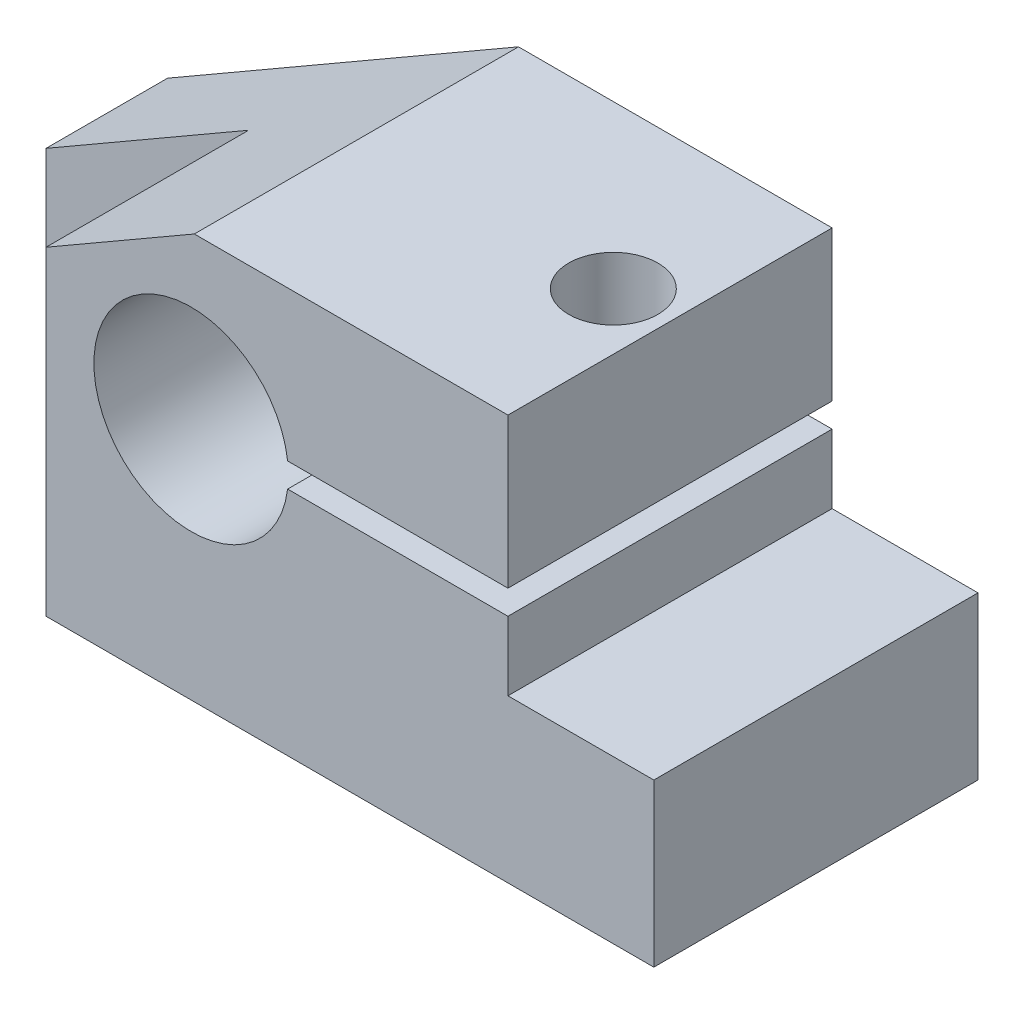
ISO-10303-21;
HEADER;
FILE_DESCRIPTION(('STEP AP214'),'2;1');
FILE_NAME('part.step','',(''),(''),'','','');
FILE_SCHEMA(('AUTOMOTIVE_DESIGN { 1 0 10303 214 1 1 1 1 }'));
ENDSEC;
DATA;
#1=APPLICATION_CONTEXT('core data for automotive mechanical design processes');
#2=APPLICATION_PROTOCOL_DEFINITION('international standard','automotive_design',2000,#1);
#3=PRODUCT_CONTEXT('',#1,'mechanical');
#4=PRODUCT('Part','Part','',(#3));
#5=PRODUCT_RELATED_PRODUCT_CATEGORY('part','',(#4));
#6=PRODUCT_DEFINITION_FORMATION('','',#4);
#7=PRODUCT_DEFINITION_CONTEXT('part definition',#1,'design');
#8=PRODUCT_DEFINITION('design','',#6,#7);
#9=PRODUCT_DEFINITION_SHAPE('','',#8);
#10=(LENGTH_UNIT() NAMED_UNIT(*) SI_UNIT(.MILLI.,.METRE.));
#11=(NAMED_UNIT(*) PLANE_ANGLE_UNIT() SI_UNIT($,.RADIAN.));
#12=(NAMED_UNIT(*) SI_UNIT($,.STERADIAN.) SOLID_ANGLE_UNIT());
#13=UNCERTAINTY_MEASURE_WITH_UNIT(LENGTH_MEASURE(1.E-05),#10,'distance_accuracy_value','');
#14=(GEOMETRIC_REPRESENTATION_CONTEXT(3) GLOBAL_UNCERTAINTY_ASSIGNED_CONTEXT((#13)) GLOBAL_UNIT_ASSIGNED_CONTEXT((#10,
#11,#12)) REPRESENTATION_CONTEXT('',''));
#15=CARTESIAN_POINT('',(0.,0.,0.));
#16=DIRECTION('',(0.,0.,1.));
#17=DIRECTION('',(1.,0.,0.));
#18=AXIS2_PLACEMENT_3D('',#15,#16,#17);
#19=CARTESIAN_POINT('',(-58.3395488539924,25.,40.));
#20=DIRECTION('',(1.,0.,0.));
#21=DIRECTION('',(0.,0.,-1.));
#22=AXIS2_PLACEMENT_3D('',#19,#20,#21);
#23=PLANE('',#22);
#24=DIRECTION('',(0.,0.,-1.));
#25=VECTOR('',#24,1.);
#26=CARTESIAN_POINT('',(-58.3395488539924,0.,40.));
#27=LINE('',#26,#25);
#28=CARTESIAN_POINT('',(-58.3395488539924,0.,15.));
#29=VERTEX_POINT('',#28);
#30=CARTESIAN_POINT('',(-58.3395488539924,0.,0.));
#31=VERTEX_POINT('',#30);
#32=EDGE_CURVE('E11',#29,#31,#27,.T.);
#33=ORIENTED_EDGE('',*,*,#32,.F.);
#34=DIRECTION('',(0.,-1.,0.));
#35=VECTOR('',#34,1.);
#36=CARTESIAN_POINT('',(-58.3395488539924,50.,15.));
#37=LINE('',#36,#35);
#38=CARTESIAN_POINT('',(-58.3395488539924,25.,15.));
#39=VERTEX_POINT('',#38);
#40=EDGE_CURVE('E257',#39,#29,#37,.T.);
#41=ORIENTED_EDGE('',*,*,#40,.F.);
#42=DIRECTION('',(0.,0.,-1.));
#43=VECTOR('',#42,1.);
#44=CARTESIAN_POINT('',(-58.3395488539924,25.,40.));
#45=LINE('',#44,#43);
#46=CARTESIAN_POINT('',(-58.3395488539924,25.,0.));
#47=VERTEX_POINT('',#46);
#48=EDGE_CURVE('E110',#39,#47,#45,.T.);
#49=ORIENTED_EDGE('',*,*,#48,.T.);
#50=DIRECTION('',(0.,-1.,0.));
#51=VECTOR('',#50,1.);
#52=CARTESIAN_POINT('',(-58.3395488539924,25.,0.));
#53=LINE('',#52,#51);
#54=EDGE_CURVE('E164',#47,#31,#53,.T.);
#55=ORIENTED_EDGE('',*,*,#54,.T.);
#56=EDGE_LOOP('',(#33,#41,#49,#55));
#57=FACE_BOUND('',#56,.T.);
#58=ADVANCED_FACE('F41',(#57),#23,.F.);
#59=CARTESIAN_POINT('',(-58.3395488539924,0.,40.));
#60=DIRECTION('',(0.,1.,0.));
#61=DIRECTION('',(0.,0.,1.));
#62=AXIS2_PLACEMENT_3D('',#59,#60,#61);
#63=PLANE('',#62);
#64=DIRECTION('',(1.,0.,0.));
#65=VECTOR('',#64,1.);
#66=CARTESIAN_POINT('',(-58.3395488539924,0.,40.));
#67=LINE('',#66,#65);
#68=CARTESIAN_POINT('',(-33.3395488539924,0.,40.));
#69=VERTEX_POINT('',#68);
#70=CARTESIAN_POINT('',(41.6604511460076,0.,40.));
#71=VERTEX_POINT('',#70);
#72=EDGE_CURVE('E113',#69,#71,#67,.T.);
#73=ORIENTED_EDGE('',*,*,#72,.F.);
#74=DIRECTION('',(0.,0.,1.));
#75=VECTOR('',#74,1.);
#76=CARTESIAN_POINT('',(-33.3395488539924,0.,15.));
#77=LINE('',#76,#75);
#78=CARTESIAN_POINT('',(-33.3395488539924,0.,15.));
#79=VERTEX_POINT('',#78);
#80=EDGE_CURVE('E57',#79,#69,#77,.T.);
#81=ORIENTED_EDGE('',*,*,#80,.F.);
#82=DIRECTION('',(1.,0.,0.));
#83=VECTOR('',#82,1.);
#84=CARTESIAN_POINT('',(-58.3395488539924,0.,15.));
#85=LINE('',#84,#83);
#86=EDGE_CURVE('E262',#29,#79,#85,.T.);
#87=ORIENTED_EDGE('',*,*,#86,.F.);
#88=ORIENTED_EDGE('',*,*,#32,.T.);
#89=DIRECTION('',(1.,0.,0.));
#90=VECTOR('',#89,1.);
#91=CARTESIAN_POINT('',(-58.3395488539924,0.,0.));
#92=LINE('',#91,#90);
#93=CARTESIAN_POINT('',(41.6604511460076,0.,0.));
#94=VERTEX_POINT('',#93);
#95=EDGE_CURVE('E170',#31,#94,#92,.T.);
#96=ORIENTED_EDGE('',*,*,#95,.T.);
#97=DIRECTION('',(0.,0.,-1.));
#98=VECTOR('',#97,1.);
#99=CARTESIAN_POINT('',(41.6604511460076,0.,40.));
#100=LINE('',#99,#98);
#101=EDGE_CURVE('E47',#71,#94,#100,.T.);
#102=ORIENTED_EDGE('',*,*,#101,.F.);
#103=EDGE_LOOP('',(#73,#81,#87,#88,#96,#102));
#104=FACE_BOUND('',#103,.T.);
#105=ADVANCED_FACE('F269',(#104),#63,.F.);
#106=CARTESIAN_POINT('',(41.6604511460076,0.,40.));
#107=DIRECTION('',(-1.,0.,0.));
#108=DIRECTION('',(0.,0.,1.));
#109=AXIS2_PLACEMENT_3D('',#106,#107,#108);
#110=PLANE('',#109);
#111=DIRECTION('',(0.,1.,0.));
#112=VECTOR('',#111,1.);
#113=CARTESIAN_POINT('',(41.6604511460076,0.,0.));
#114=LINE('',#113,#112);
#115=CARTESIAN_POINT('',(41.6604511460076,20.,0.));
#116=VERTEX_POINT('',#115);
#117=EDGE_CURVE('E168',#94,#116,#114,.T.);
#118=ORIENTED_EDGE('',*,*,#117,.T.);
#119=DIRECTION('',(0.,0.,-1.));
#120=VECTOR('',#119,1.);
#121=CARTESIAN_POINT('',(41.6604511460076,20.,40.));
#122=LINE('',#121,#120);
#123=CARTESIAN_POINT('',(41.6604511460076,20.,40.));
#124=VERTEX_POINT('',#123);
#125=EDGE_CURVE('E204',#124,#116,#122,.T.);
#126=ORIENTED_EDGE('',*,*,#125,.F.);
#127=DIRECTION('',(0.,1.,0.));
#128=VECTOR('',#127,1.);
#129=CARTESIAN_POINT('',(41.6604511460076,0.,40.));
#130=LINE('',#129,#128);
#131=EDGE_CURVE('E213',#71,#124,#130,.T.);
#132=ORIENTED_EDGE('',*,*,#131,.F.);
#133=ORIENTED_EDGE('',*,*,#101,.T.);
#134=EDGE_LOOP('',(#118,#126,#132,#133));
#135=FACE_BOUND('',#134,.T.);
#136=ADVANCED_FACE('F211',(#135),#110,.F.);
#137=CARTESIAN_POINT('',(41.6604511460076,20.,40.));
#138=DIRECTION('',(0.,-1.,0.));
#139=DIRECTION('',(0.,0.,-1.));
#140=AXIS2_PLACEMENT_3D('',#137,#138,#139);
#141=PLANE('',#140);
#142=DIRECTION('',(-1.,0.,0.));
#143=VECTOR('',#142,1.);
#144=CARTESIAN_POINT('',(41.6604511460076,20.,0.));
#145=LINE('',#144,#143);
#146=CARTESIAN_POINT('',(23.6604511460076,20.,0.));
#147=VERTEX_POINT('',#146);
#148=EDGE_CURVE('E175',#116,#147,#145,.T.);
#149=ORIENTED_EDGE('',*,*,#148,.T.);
#150=DIRECTION('',(0.,0.,-1.));
#151=VECTOR('',#150,1.);
#152=CARTESIAN_POINT('',(23.6604511460076,20.,40.));
#153=LINE('',#152,#151);
#154=CARTESIAN_POINT('',(23.6604511460076,20.,40.));
#155=VERTEX_POINT('',#154);
#156=EDGE_CURVE('E203',#155,#147,#153,.T.);
#157=ORIENTED_EDGE('',*,*,#156,.F.);
#158=DIRECTION('',(-1.,0.,0.));
#159=VECTOR('',#158,1.);
#160=CARTESIAN_POINT('',(41.6604511460076,20.,40.));
#161=LINE('',#160,#159);
#162=EDGE_CURVE('E232',#124,#155,#161,.T.);
#163=ORIENTED_EDGE('',*,*,#162,.F.);
#164=ORIENTED_EDGE('',*,*,#125,.T.);
#165=EDGE_LOOP('',(#149,#157,#163,#164));
#166=FACE_BOUND('',#165,.T.);
#167=ADVANCED_FACE('F224',(#166),#141,.F.);
#168=CARTESIAN_POINT('',(23.6604511460076,20.,40.));
#169=DIRECTION('',(-1.,0.,0.));
#170=DIRECTION('',(0.,0.,1.));
#171=AXIS2_PLACEMENT_3D('',#168,#169,#170);
#172=PLANE('',#171);
#173=DIRECTION('',(0.,1.,0.));
#174=VECTOR('',#173,1.);
#175=CARTESIAN_POINT('',(23.6604511460076,20.,0.));
#176=LINE('',#175,#174);
#177=CARTESIAN_POINT('',(23.6604511460076,28.5,0.));
#178=VERTEX_POINT('',#177);
#179=EDGE_CURVE('E174',#147,#178,#176,.T.);
#180=ORIENTED_EDGE('',*,*,#179,.T.);
#181=DIRECTION('',(0.,0.,-1.));
#182=VECTOR('',#181,1.);
#183=CARTESIAN_POINT('',(23.6604511460076,28.5,40.));
#184=LINE('',#183,#182);
#185=CARTESIAN_POINT('',(23.6604511460076,28.5,40.));
#186=VERTEX_POINT('',#185);
#187=EDGE_CURVE('E196',#186,#178,#184,.T.);
#188=ORIENTED_EDGE('',*,*,#187,.F.);
#189=DIRECTION('',(0.,1.,0.));
#190=VECTOR('',#189,1.);
#191=CARTESIAN_POINT('',(23.6604511460076,20.,40.));
#192=LINE('',#191,#190);
#193=EDGE_CURVE('E229',#155,#186,#192,.T.);
#194=ORIENTED_EDGE('',*,*,#193,.F.);
#195=ORIENTED_EDGE('',*,*,#156,.T.);
#196=EDGE_LOOP('',(#180,#188,#194,#195));
#197=FACE_BOUND('',#196,.T.);
#198=ADVANCED_FACE('F230',(#197),#172,.F.);
#199=CARTESIAN_POINT('',(23.6604511460076,28.5,40.));
#200=DIRECTION('',(0.,-1.,0.));
#201=DIRECTION('',(1.,0.,0.));
#202=AXIS2_PLACEMENT_3D('',#199,#200,#201);
#203=PLANE('',#202);
#204=DIRECTION('',(-1.,0.,0.));
#205=VECTOR('',#204,1.);
#206=CARTESIAN_POINT('',(23.6604511460076,28.5,0.));
#207=LINE('',#206,#205);
#208=CARTESIAN_POINT('',(-3.52361977982805,28.5,0.));
#209=VERTEX_POINT('',#208);
#210=EDGE_CURVE('E176',#178,#209,#207,.T.);
#211=ORIENTED_EDGE('',*,*,#210,.T.);
#212=DIRECTION('',(0.,0.,-1.));
#213=VECTOR('',#212,1.);
#214=CARTESIAN_POINT('',(-3.52361977982805,28.5,40.));
#215=LINE('',#214,#213);
#216=CARTESIAN_POINT('',(-3.52361977982805,28.5,40.));
#217=VERTEX_POINT('',#216);
#218=EDGE_CURVE('E198',#217,#209,#215,.T.);
#219=ORIENTED_EDGE('',*,*,#218,.F.);
#220=DIRECTION('',(-1.,0.,0.));
#221=VECTOR('',#220,1.);
#222=CARTESIAN_POINT('',(23.6604511460076,28.5,40.));
#223=LINE('',#222,#221);
#224=EDGE_CURVE('E231',#186,#217,#223,.T.);
#225=ORIENTED_EDGE('',*,*,#224,.F.);
#226=ORIENTED_EDGE('',*,*,#187,.T.);
#227=EDGE_LOOP('',(#211,#219,#225,#226));
#228=FACE_BOUND('',#227,.T.);
#229=ADVANCED_FACE('F313',(#228),#203,.F.);
#230=CARTESIAN_POINT('',(-15.4295006796187,30.,40.));
#231=DIRECTION('',(0.,0.,-1.));
#232=DIRECTION('',(-1.,0.,0.));
#233=AXIS2_PLACEMENT_3D('',#230,#231,#232);
#234=CYLINDRICAL_SURFACE('',#233,12.);
#235=CARTESIAN_POINT('',(-15.4295006796187,30.,0.));
#236=DIRECTION('',(0.,0.,1.));
#237=DIRECTION('',(1.,0.,0.));
#238=AXIS2_PLACEMENT_3D('',#235,#236,#237);
#239=CIRCLE('',#238,12.);
#240=CARTESIAN_POINT('',(-3.52361977982805,31.5,0.));
#241=VERTEX_POINT('',#240);
#242=EDGE_CURVE('E178',#241,#209,#239,.T.);
#243=ORIENTED_EDGE('',*,*,#242,.F.);
#244=DIRECTION('',(0.,0.,-1.));
#245=VECTOR('',#244,1.);
#246=CARTESIAN_POINT('',(-3.52361977982805,31.5,40.));
#247=LINE('',#246,#245);
#248=CARTESIAN_POINT('',(-3.52361977982805,31.5,40.));
#249=VERTEX_POINT('',#248);
#250=EDGE_CURVE('E152',#249,#241,#247,.T.);
#251=ORIENTED_EDGE('',*,*,#250,.F.);
#252=CARTESIAN_POINT('',(-15.4295006796187,30.,40.));
#253=DIRECTION('',(0.,0.,1.));
#254=DIRECTION('',(1.,0.,0.));
#255=AXIS2_PLACEMENT_3D('',#252,#253,#254);
#256=CIRCLE('',#255,12.);
#257=EDGE_CURVE('E141',#249,#217,#256,.T.);
#258=ORIENTED_EDGE('',*,*,#257,.T.);
#259=ORIENTED_EDGE('',*,*,#218,.T.);
#260=EDGE_LOOP('',(#243,#251,#258,#259));
#261=FACE_BOUND('',#260,.T.);
#262=ADVANCED_FACE('F239',(#261),#234,.F.);
#263=CARTESIAN_POINT('',(-3.52361977982805,31.5,40.));
#264=DIRECTION('',(0.,1.,0.));
#265=DIRECTION('',(0.,0.,1.));
#266=AXIS2_PLACEMENT_3D('',#263,#264,#265);
#267=PLANE('',#266);
#268=CARTESIAN_POINT('',(16.6604511460076,31.5,20.));
#269=DIRECTION('',(0.,1.,0.));
#270=DIRECTION('',(0.,0.,1.));
#271=AXIS2_PLACEMENT_3D('',#268,#269,#270);
#272=CIRCLE('',#271,5.5);
#273=CARTESIAN_POINT('',(16.6604511460076,31.5,25.5));
#274=VERTEX_POINT('',#273);
#275=EDGE_CURVE('E271',#274,#274,#272,.F.);
#276=ORIENTED_EDGE('',*,*,#275,.F.);
#277=EDGE_LOOP('',(#276));
#278=FACE_BOUND('',#277,.T.);
#279=DIRECTION('',(1.,0.,0.));
#280=VECTOR('',#279,1.);
#281=CARTESIAN_POINT('',(-3.52361977982805,31.5,0.));
#282=LINE('',#281,#280);
#283=CARTESIAN_POINT('',(23.6604511460076,31.5,0.));
#284=VERTEX_POINT('',#283);
#285=EDGE_CURVE('E147',#241,#284,#282,.T.);
#286=ORIENTED_EDGE('',*,*,#285,.T.);
#287=DIRECTION('',(0.,0.,-1.));
#288=VECTOR('',#287,1.);
#289=CARTESIAN_POINT('',(23.6604511460076,31.5,40.));
#290=LINE('',#289,#288);
#291=CARTESIAN_POINT('',(23.6604511460076,31.5,40.));
#292=VERTEX_POINT('',#291);
#293=EDGE_CURVE('E150',#292,#284,#290,.T.);
#294=ORIENTED_EDGE('',*,*,#293,.F.);
#295=DIRECTION('',(1.,0.,0.));
#296=VECTOR('',#295,1.);
#297=CARTESIAN_POINT('',(-3.52361977982805,31.5,40.));
#298=LINE('',#297,#296);
#299=EDGE_CURVE('E132',#249,#292,#298,.T.);
#300=ORIENTED_EDGE('',*,*,#299,.F.);
#301=ORIENTED_EDGE('',*,*,#250,.T.);
#302=EDGE_LOOP('',(#286,#294,#300,#301));
#303=FACE_BOUND('',#302,.T.);
#304=ADVANCED_FACE('F146',(#278,#303),#267,.F.);
#305=CARTESIAN_POINT('',(23.6604511460076,31.5,40.));
#306=DIRECTION('',(-1.,0.,0.));
#307=DIRECTION('',(0.,0.,1.));
#308=AXIS2_PLACEMENT_3D('',#305,#306,#307);
#309=PLANE('',#308);
#310=DIRECTION('',(0.,1.,0.));
#311=VECTOR('',#310,1.);
#312=CARTESIAN_POINT('',(23.6604511460076,31.5,0.));
#313=LINE('',#312,#311);
#314=CARTESIAN_POINT('',(23.6604511460076,50.,0.));
#315=VERTEX_POINT('',#314);
#316=EDGE_CURVE('E181',#284,#315,#313,.T.);
#317=ORIENTED_EDGE('',*,*,#316,.T.);
#318=DIRECTION('',(0.,0.,-1.));
#319=VECTOR('',#318,1.);
#320=CARTESIAN_POINT('',(23.6604511460076,50.,40.));
#321=LINE('',#320,#319);
#322=CARTESIAN_POINT('',(23.6604511460076,50.,40.));
#323=VERTEX_POINT('',#322);
#324=EDGE_CURVE('E154',#323,#315,#321,.T.);
#325=ORIENTED_EDGE('',*,*,#324,.F.);
#326=DIRECTION('',(0.,1.,0.));
#327=VECTOR('',#326,1.);
#328=CARTESIAN_POINT('',(23.6604511460076,31.5,40.));
#329=LINE('',#328,#327);
#330=EDGE_CURVE('E140',#292,#323,#329,.T.);
#331=ORIENTED_EDGE('',*,*,#330,.F.);
#332=ORIENTED_EDGE('',*,*,#293,.T.);
#333=EDGE_LOOP('',(#317,#325,#331,#332));
#334=FACE_BOUND('',#333,.T.);
#335=ADVANCED_FACE('F160',(#334),#309,.F.);
#336=CARTESIAN_POINT('',(-15.0382786647703,50.,40.));
#337=DIRECTION('',(0.,1.,0.));
#338=DIRECTION('',(0.,0.,1.));
#339=AXIS2_PLACEMENT_3D('',#336,#337,#338);
#340=PLANE('',#339);
#341=CARTESIAN_POINT('',(16.6604511460076,50.,20.));
#342=DIRECTION('',(0.,1.,0.));
#343=DIRECTION('',(0.,0.,1.));
#344=AXIS2_PLACEMENT_3D('',#341,#342,#343);
#345=CIRCLE('',#344,5.5);
#346=CARTESIAN_POINT('',(16.6604511460076,50.,25.5));
#347=VERTEX_POINT('',#346);
#348=EDGE_CURVE('E435',#347,#347,#345,.T.);
#349=ORIENTED_EDGE('',*,*,#348,.F.);
#350=EDGE_LOOP('',(#349));
#351=FACE_BOUND('',#350,.T.);
#352=DIRECTION('',(1.,0.,0.));
#353=VECTOR('',#352,1.);
#354=CARTESIAN_POINT('',(-15.0382786647703,50.,0.));
#355=LINE('',#354,#353);
#356=CARTESIAN_POINT('',(-15.0382786647703,50.,0.));
#357=VERTEX_POINT('',#356);
#358=EDGE_CURVE('E183',#357,#315,#355,.T.);
#359=ORIENTED_EDGE('',*,*,#358,.F.);
#360=DIRECTION('',(0.,0.,-1.));
#361=VECTOR('',#360,1.);
#362=CARTESIAN_POINT('',(-15.0382786647703,50.,40.));
#363=LINE('',#362,#361);
#364=CARTESIAN_POINT('',(-15.0382786647703,50.,40.));
#365=VERTEX_POINT('',#364);
#366=EDGE_CURVE('E192',#365,#357,#363,.T.);
#367=ORIENTED_EDGE('',*,*,#366,.F.);
#368=DIRECTION('',(1.,0.,0.));
#369=VECTOR('',#368,1.);
#370=CARTESIAN_POINT('',(-15.0382786647703,50.,40.));
#371=LINE('',#370,#369);
#372=EDGE_CURVE('E157',#365,#323,#371,.T.);
#373=ORIENTED_EDGE('',*,*,#372,.T.);
#374=ORIENTED_EDGE('',*,*,#324,.T.);
#375=EDGE_LOOP('',(#359,#367,#373,#374));
#376=FACE_BOUND('',#375,.T.);
#377=ADVANCED_FACE('F244',(#351,#376),#340,.T.);
#378=CARTESIAN_POINT('',(-58.3395488539924,25.,40.));
#379=DIRECTION('',(-0.499999999999998,0.86602540378444,0.));
#380=DIRECTION('',(-0.86602540378444,-0.499999999999998,0.));
#381=AXIS2_PLACEMENT_3D('',#378,#379,#380);
#382=PLANE('',#381);
#383=DIRECTION('',(0.,0.,-1.));
#384=VECTOR('',#383,1.);
#385=CARTESIAN_POINT('',(-33.3395488539924,39.4337567297406,40.));
#386=LINE('',#385,#384);
#387=CARTESIAN_POINT('',(-33.3395488539924,39.4337567297406,40.));
#388=VERTEX_POINT('',#387);
#389=CARTESIAN_POINT('',(-33.3395488539924,39.4337567297406,15.));
#390=VERTEX_POINT('',#389);
#391=EDGE_CURVE('E248',#388,#390,#386,.T.);
#392=ORIENTED_EDGE('',*,*,#391,.F.);
#393=DIRECTION('',(0.86602540378444,0.499999999999998,0.));
#394=VECTOR('',#393,1.);
#395=CARTESIAN_POINT('',(-58.3395488539924,25.,40.));
#396=LINE('',#395,#394);
#397=EDGE_CURVE('E62',#388,#365,#396,.T.);
#398=ORIENTED_EDGE('',*,*,#397,.T.);
#399=ORIENTED_EDGE('',*,*,#366,.T.);
#400=DIRECTION('',(0.86602540378444,0.499999999999998,0.));
#401=VECTOR('',#400,1.);
#402=CARTESIAN_POINT('',(-58.3395488539924,25.,0.));
#403=LINE('',#402,#401);
#404=EDGE_CURVE('E186',#47,#357,#403,.T.);
#405=ORIENTED_EDGE('',*,*,#404,.F.);
#406=ORIENTED_EDGE('',*,*,#48,.F.);
#407=DIRECTION('',(-0.86602540378444,-0.499999999999998,0.));
#408=VECTOR('',#407,1.);
#409=CARTESIAN_POINT('',(-58.3395488539924,25.,15.));
#410=LINE('',#409,#408);
#411=EDGE_CURVE('E266',#390,#39,#410,.T.);
#412=ORIENTED_EDGE('',*,*,#411,.F.);
#413=EDGE_LOOP('',(#392,#398,#399,#405,#406,#412));
#414=FACE_BOUND('',#413,.T.);
#415=ADVANCED_FACE('F272',(#414),#382,.T.);
#416=CARTESIAN_POINT('',(-15.4295006796187,30.,40.));
#417=DIRECTION('',(0.,0.,1.));
#418=DIRECTION('',(1.,0.,0.));
#419=AXIS2_PLACEMENT_3D('',#416,#417,#418);
#420=PLANE('',#419);
#421=DIRECTION('',(0.,-1.,0.));
#422=VECTOR('',#421,1.);
#423=CARTESIAN_POINT('',(-33.3395488539924,50.,40.));
#424=LINE('',#423,#422);
#425=EDGE_CURVE('E242',#388,#69,#424,.T.);
#426=ORIENTED_EDGE('',*,*,#425,.T.);
#427=ORIENTED_EDGE('',*,*,#72,.T.);
#428=ORIENTED_EDGE('',*,*,#131,.T.);
#429=ORIENTED_EDGE('',*,*,#162,.T.);
#430=ORIENTED_EDGE('',*,*,#193,.T.);
#431=ORIENTED_EDGE('',*,*,#224,.T.);
#432=ORIENTED_EDGE('',*,*,#257,.F.);
#433=ORIENTED_EDGE('',*,*,#299,.T.);
#434=ORIENTED_EDGE('',*,*,#330,.T.);
#435=ORIENTED_EDGE('',*,*,#372,.F.);
#436=ORIENTED_EDGE('',*,*,#397,.F.);
#437=EDGE_LOOP('',(#426,#427,#428,#429,#430,#431,#432,#433,#434,#435,#436));
#438=FACE_BOUND('',#437,.T.);
#439=ADVANCED_FACE('F137',(#438),#420,.T.);
#440=CARTESIAN_POINT('',(-15.4295006796187,30.,0.));
#441=DIRECTION('',(0.,0.,1.));
#442=DIRECTION('',(1.,0.,0.));
#443=AXIS2_PLACEMENT_3D('',#440,#441,#442);
#444=PLANE('',#443);
#445=CARTESIAN_POINT('',(-45.3395488539924,12.,0.));
#446=DIRECTION('',(0.,0.,1.));
#447=DIRECTION('',(1.,0.,0.));
#448=AXIS2_PLACEMENT_3D('',#445,#446,#447);
#449=CIRCLE('',#448,4.5);
#450=CARTESIAN_POINT('',(-40.8395488539924,12.,0.));
#451=VERTEX_POINT('',#450);
#452=EDGE_CURVE('E169',#451,#451,#449,.T.);
#453=ORIENTED_EDGE('',*,*,#452,.T.);
#454=EDGE_LOOP('',(#453));
#455=FACE_BOUND('',#454,.T.);
#456=ORIENTED_EDGE('',*,*,#54,.F.);
#457=ORIENTED_EDGE('',*,*,#404,.T.);
#458=ORIENTED_EDGE('',*,*,#358,.T.);
#459=ORIENTED_EDGE('',*,*,#316,.F.);
#460=ORIENTED_EDGE('',*,*,#285,.F.);
#461=ORIENTED_EDGE('',*,*,#242,.T.);
#462=ORIENTED_EDGE('',*,*,#210,.F.);
#463=ORIENTED_EDGE('',*,*,#179,.F.);
#464=ORIENTED_EDGE('',*,*,#148,.F.);
#465=ORIENTED_EDGE('',*,*,#117,.F.);
#466=ORIENTED_EDGE('',*,*,#95,.F.);
#467=EDGE_LOOP('',(#456,#457,#458,#459,#460,#461,#462,#463,#464,#465,#466));
#468=FACE_BOUND('',#467,.T.);
#469=ADVANCED_FACE('F217',(#455,#468),#444,.F.);
#470=CARTESIAN_POINT('',(-45.3395488539924,12.,0.));
#471=DIRECTION('',(0.,0.,1.));
#472=DIRECTION('',(1.,0.,0.));
#473=AXIS2_PLACEMENT_3D('',#470,#471,#472);
#474=CYLINDRICAL_SURFACE('',#473,4.5);
#475=CARTESIAN_POINT('',(-45.3395488539924,12.,15.));
#476=DIRECTION('',(0.,0.,-1.));
#477=DIRECTION('',(-1.,0.,0.));
#478=AXIS2_PLACEMENT_3D('',#475,#476,#477);
#479=CIRCLE('',#478,4.5);
#480=CARTESIAN_POINT('',(-49.8395488539924,12.,15.));
#481=VERTEX_POINT('',#480);
#482=EDGE_CURVE('E42',#481,#481,#479,.F.);
#483=ORIENTED_EDGE('',*,*,#482,.T.);
#484=EDGE_LOOP('',(#483));
#485=FACE_BOUND('',#484,.T.);
#486=ORIENTED_EDGE('',*,*,#452,.F.);
#487=EDGE_LOOP('',(#486));
#488=FACE_BOUND('',#487,.T.);
#489=ADVANCED_FACE('F284',(#485,#488),#474,.F.);
#490=CARTESIAN_POINT('',(-58.3395488539924,50.,15.));
#491=DIRECTION('',(0.,0.,-1.));
#492=DIRECTION('',(-1.,0.,0.));
#493=AXIS2_PLACEMENT_3D('',#490,#491,#492);
#494=PLANE('',#493);
#495=ORIENTED_EDGE('',*,*,#411,.T.);
#496=ORIENTED_EDGE('',*,*,#40,.T.);
#497=ORIENTED_EDGE('',*,*,#86,.T.);
#498=DIRECTION('',(0.,-1.,0.));
#499=VECTOR('',#498,1.);
#500=CARTESIAN_POINT('',(-33.3395488539924,50.,15.));
#501=LINE('',#500,#499);
#502=EDGE_CURVE('E268',#390,#79,#501,.T.);
#503=ORIENTED_EDGE('',*,*,#502,.F.);
#504=EDGE_LOOP('',(#495,#496,#497,#503));
#505=FACE_BOUND('',#504,.T.);
#506=ORIENTED_EDGE('',*,*,#482,.F.);
#507=EDGE_LOOP('',(#506));
#508=FACE_BOUND('',#507,.T.);
#509=ADVANCED_FACE('F265',(#505,#508),#494,.F.);
#510=CARTESIAN_POINT('',(-33.3395488539924,50.,15.));
#511=DIRECTION('',(1.,0.,0.));
#512=DIRECTION('',(0.,0.,-1.));
#513=AXIS2_PLACEMENT_3D('',#510,#511,#512);
#514=PLANE('',#513);
#515=ORIENTED_EDGE('',*,*,#391,.T.);
#516=ORIENTED_EDGE('',*,*,#502,.T.);
#517=ORIENTED_EDGE('',*,*,#80,.T.);
#518=ORIENTED_EDGE('',*,*,#425,.F.);
#519=EDGE_LOOP('',(#515,#516,#517,#518));
#520=FACE_BOUND('',#519,.T.);
#521=ADVANCED_FACE('F295',(#520),#514,.F.);
#522=CARTESIAN_POINT('',(16.6604511460076,15.943650813896,20.));
#523=DIRECTION('',(0.,1.,0.));
#524=DIRECTION('',(0.,0.,1.));
#525=AXIS2_PLACEMENT_3D('',#522,#523,#524);
#526=CYLINDRICAL_SURFACE('',#525,5.5);
#527=ORIENTED_EDGE('',*,*,#275,.T.);
#528=EDGE_LOOP('',(#527));
#529=FACE_BOUND('',#528,.T.);
#530=ORIENTED_EDGE('',*,*,#348,.T.);
#531=EDGE_LOOP('',(#530));
#532=FACE_BOUND('',#531,.T.);
#533=ADVANCED_FACE('F397',(#529,#532),#526,.F.);
#534=CLOSED_SHELL('',(#58,#105,#136,#167,#198,#229,#262,#304,#335,#377,#415,#439,#469,#489,#509,
#521,#533));
#535=MANIFOLD_SOLID_BREP('B2',#534);
#536=ADVANCED_BREP_SHAPE_REPRESENTATION('',(#18,#535),#14);
#537=SHAPE_DEFINITION_REPRESENTATION(#9,#536);
ENDSEC;
END-ISO-10303-21;
